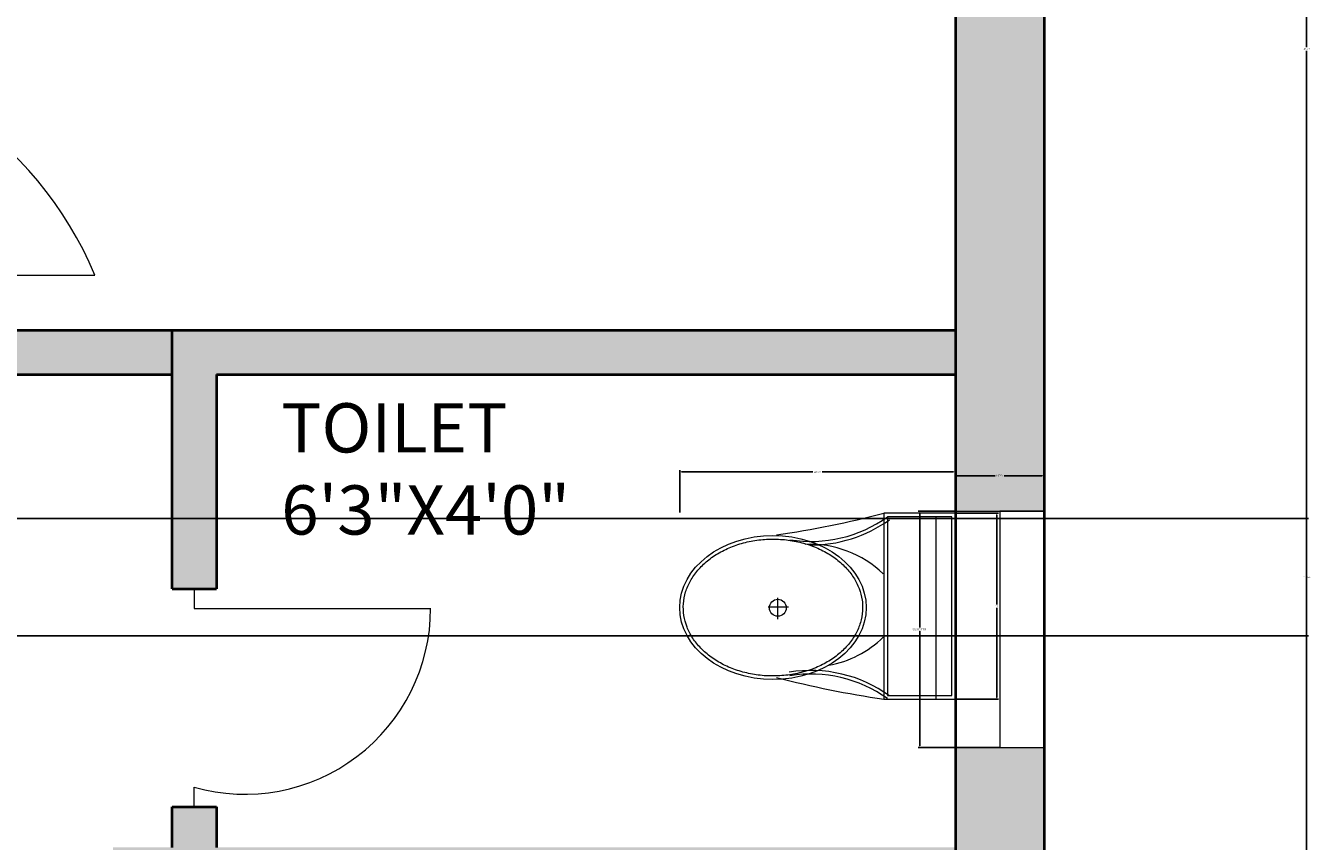
# Model space of a CAD drawing. Units: inches. Extents: x 1441 to 2460, y 1648 to 2683.
# Tile 14 of 35: x 1786 to 1916, y 1975 to 2058. Entities that reach past the tile are written whole.
import ezdxf

# ---------------------------------------------------------------- set-up
doc = ezdxf.new("R2010")
doc.units = ezdxf.units.IN
for name, color, linetype, lineweight in [('A-ANNO-DIMS', 2, 'Continuous', 18), ('A-AREA-IDEN', 7, 'Continuous', 20), ('A-DOOR', 3, 'Continuous', 20), ('A-FLOR-FIXT', 9, 'Continuous', 18), ('A-GLAZ', 4, 'Continuous', 18), ('A-WALL', 7, 'Continuous', 40)]:
    doc.layers.add(name, color=color, linetype=linetype, lineweight=lineweight)
doc.layers.add('A-WALL-PATT', color=251, linetype='Continuous', lineweight=13, true_color=0x636466)
doc.styles.get("Standard").update_dxf_attribs({"font": 'arial.ttf'})
doc.dimstyles.get("Standard").update_dxf_attribs({"dimtxt": 0.18, "dimasz": 0.18, "dimexe": 0.18, "dimexo": 0.0625, "dimgap": 0.09, "dimtad": 0, "dimtih": 1, "dimtoh": 1, "dimdec": 4, "dimzin": 0, "dimdsep": 46, "dimtxsty": 'Standard', "dimcen": 0.09, "dimadec": 0, "dimazin": 0, "dimtfac": 1, "dimtdec": 4, "dimtofl": 0, "dimtmove": 0, "dimatfit": 3, "dimfxl": 1, "dimtolj": 1, "dimtzin": 0, "dimarcsym": 0})

# ---------------------------------------------------------------- blocks, each defined once
blk = doc.blocks.new('A$C31115884')
for p, q in [((257.5, 466.4), (257.5, 523.2)), ((283.1, 497.7), (223.4, 497.7)), ((0, 200), (0, 0)), ((520, 200), (0, 200)), ((10, 190), (10, 10)), ((510, 190), (10, 190)), ((510, 10), (510, 190)), ((520, 0), (520, 200)), ((510, 54.5), (0, 54.5)), ((10, 10), (510, 10)), ((0, 0), (520, 0))]:
    blk.add_line(p, q)
blk.add_circle((255.6, 496.4), 23.6)
for centre, radius, start, end in [((2777.7, -204.6), 2807, 165.4549, 171.7133), ((3237, 905), 2807, 188.2867, 194.5451), ((-294.5, 403.3), 364.7, 324.2091, 9.3499), ((-294.5, 403.3), 374.7, 324.2091, 9.3499), ((805.8, 403.3), 364.7, 170.6501, 215.7909), ((139.5, 406.2), 293.5, 315.8436, 2.6563), ((805.8, 403.3), 374.7, 179.2036, 215.7909), ((383.6, 406.2), 293.5, 190.2774, 224.1564)]:
    blk.add_arc(centre, radius, start, end)
blk.add_ellipse((256.2, 509.9), major_axis=(0, -260.7), ratio=0.772727)
blk.add_open_spline([(256.2, 259.2), (263.1, 259.2), (270, 259.7), (287.8, 262.3), (298.7, 265.1), (319.9, 273.1), (330.2, 278.4), (350.1, 291.1), (359.7, 298.7), (377.7, 315.9), (386.2, 325.5), (401.7, 346.6), (408.8, 358.1), (421.3, 382.5), (426.8, 395.5), (435.9, 422.4), (439.5, 436.4), (444.8, 465.1), (446.5, 479.7), (447.9, 509.2), (447.6, 524), (445, 553.3), (442.7, 567.8), (436.3, 596), (432.1, 609.7), (421.9, 636), (416, 648.6), (402.5, 672.1), (395, 683), (378.6, 703), (369.8, 712.1), (351.1, 728), (341.3, 734.8), (320.9, 746.2), (310.4, 750.7), (288.9, 757.3), (278, 759.4), (256, 761), (245, 760.6), (223.1, 757.2), (212.3, 754.3), (191.1, 746.1), (180.8, 740.7), (160.9, 727.8), (151.4, 720.1), (133.5, 702.7), (125.1, 693), (109.6, 671.7), (102.6, 660.2), (90.2, 635.7), (84.9, 622.7), (76, 595.6), (72.4, 581.6), (67.2, 552.9), (65.6, 538.2), (64.4, 508.8), (64.8, 494), (67.5, 464.7), (69.9, 450.2), (76.6, 422), (80.8, 408.3), (91.1, 382.2), (97.2, 369.7), (110.8, 346.3), (118.4, 335.4), (134.8, 315.6), (143.7, 306.7), (162.4, 290.9), (172.3, 284.2), (192.8, 273), (203.3, 268.6), (224.8, 262.2), (235.8, 260.2), (249.9, 259.3), (253, 259.2), (256.2, 259.2)], degree=3, knots=[0, 0, 0, 0, 0.110105, 0.110105, 0.285049, 0.285049, 0.459994, 0.459994, 0.634938, 0.634938, 0.809882, 0.809882, 0.984827, 0.984827, 1.159771, 1.159771, 1.334715, 1.334715, 1.50966, 1.50966, 1.684604, 1.684604, 1.859549, 1.859549, 2.034493, 2.034493, 2.209437, 2.209437, 2.384382, 2.384382, 2.559326, 2.559326, 2.73427, 2.73427, 2.909215, 2.909215, 3.084159, 3.084159, 3.259103, 3.259103, 3.434048, 3.434048, 3.608992, 3.608992, 3.783936, 3.783936, 3.958881, 3.958881, 4.133825, 4.133825, 4.30877, 4.30877, 4.483714, 4.483714, 4.658658, 4.658658, 4.833603, 4.833603, 5.008547, 5.008547, 5.183491, 5.183491, 5.358436, 5.358436, 5.53338, 5.53338, 5.708324, 5.708324, 5.883269, 5.883269, 6.058213, 6.058213, 6.233158, 6.233158, 6.283185, 6.283185, 6.283185, 6.283185])
blk = doc.blocks.new('DOOR-BED2-30')
for p, q in [((0, 27.22), (0, 25.22)), ((0, 0), (0, 2)), ((0, 2), (4.91, 2)), ((4.91, 2), (34.91, 2))]:
    blk.add_line(p, q)
blk.add_arc((0, -12.65), 37.87, 22.7676, 90)
blk = doc.blocks.new('DOOR-WC-SOUTH-24')
for p, q in [((0, 22.15), (0, 20.15)), ((0, 20.15), (24, 20.15)), ((0, 0), (0, 2))]:
    blk.add_line(p, q)
blk.add_arc((5.13, 20.15), 18.86, 254.1904, 0)
blk = doc.blocks.new('WIN-24-SASH')
for p, q in [((9, 24), (4.5, 24)), ((4.5, 24), (4.5, 0)), ((4.5, 0), (0, 0))]:
    blk.add_line(p, q)
blk = doc.blocks.new('*D32')
at = {"layer": 'A-ANNO-DIMS', "color": 0, "lineweight": -2, "transparency": 16777216}
for p, q in [((1852.41, 2008.68), (1852.41, 2013)), ((1852.59, 2012.82), (1865.93, 2012.82)), ((1880.21, 2012.82), (1866.87, 2012.82)), ((1880.39, 2008.68), (1880.39, 2013))]:
    blk.add_line(p, q, dxfattribs=at)
at = {"layer": 'A-ANNO-DIMS', "color": 0, "transparency": 16777216}
for points in [[(1852.59, 2012.85), (1852.59, 2012.79), (1852.41, 2012.82)], [(1880.21, 2012.85), (1880.21, 2012.79), (1880.39, 2012.82)]]:
    blk.add_solid(points, dxfattribs=at)
at = {"layer": 'Defpoints', "color": 0, "transparency": 16777216}
for p in [(1852.41, 2012.82), (1852.41, 2008.62), (1880.39, 2008.62)]:
    blk.add_point(p, dxfattribs=at)
at = {"layer": 'A-ANNO-DIMS', "color": 0, "transparency": 16777216, "insert": (1866.4, 2012.82), "char_height": 0.18, "attachment_point": 5}
blk.add_mtext('\\A1;WC 28', dxfattribs=at)
blk = doc.blocks.new('*D33')
at = {"layer": 'A-ANNO-DIMS', "color": 0, "lineweight": -2, "transparency": 16777216}
for p, q in [((1880.45, 2008.62), (1884.76, 2008.62)), ((1884.58, 2008.44), (1884.58, 1999.36)), ((1884.58, 1989.92), (1884.58, 1999)), ((1880.45, 1989.74), (1884.76, 1989.74))]:
    blk.add_line(p, q, dxfattribs=at)
at = {"layer": 'A-ANNO-DIMS', "color": 0, "transparency": 16777216}
for points in [[(1884.55, 2008.44), (1884.61, 2008.44), (1884.58, 2008.62)], [(1884.55, 1989.92), (1884.61, 1989.92), (1884.58, 1989.74)]]:
    blk.add_solid(points, dxfattribs=at)
at = {"layer": 'Defpoints', "color": 0, "transparency": 16777216}
for p in [(1880.39, 2008.62), (1884.58, 2008.62), (1880.39, 1989.74)]:
    blk.add_point(p, dxfattribs=at)
at = {"layer": 'A-ANNO-DIMS', "color": 0, "transparency": 16777216, "insert": (1884.58, 1999.18), "char_height": 0.18, "attachment_point": 5}
blk.add_mtext('\\A1;19', dxfattribs=at)
blk = doc.blocks.new('*D60')
at = {"layer": 'A-ANNO-DIMS', "color": 0, "lineweight": -2, "transparency": 16777216}
for p, q in [((1880.32, 2008.83), (1876.61, 2008.83)), ((1876.79, 2008.65), (1876.79, 1997.01)), ((1876.79, 1985.01), (1876.79, 1996.65)), ((1880.32, 1984.83), (1876.61, 1984.83))]:
    blk.add_line(p, q, dxfattribs=at)
at = {"layer": 'A-ANNO-DIMS', "color": 0, "transparency": 16777216}
for points in [[(1876.76, 2008.65), (1876.82, 2008.65), (1876.79, 2008.83)], [(1876.76, 1985.01), (1876.82, 1985.01), (1876.79, 1984.83)]]:
    blk.add_solid(points, dxfattribs=at)
at = {"layer": 'Defpoints', "color": 0, "transparency": 16777216}
for p in [(1876.79, 2008.83), (1880.39, 2008.83), (1880.39, 1984.83)]:
    blk.add_point(p, dxfattribs=at)
at = {"layer": 'A-ANNO-DIMS', "color": 0, "transparency": 16777216, "insert": (1876.79, 1996.83), "char_height": 0.18, "attachment_point": 5}
blk.add_mtext('\\A1;SASH 24 TYP.', dxfattribs=at)
blk = doc.blocks.new('*D61')
at = {"layer": 'A-ANNO-DIMS', "color": 0, "lineweight": -2, "transparency": 16777216}
for p, q in [((1880.39, 2008.89), (1880.39, 2012.61)), ((1880.57, 2012.43), (1884.43, 2012.43)), ((1889.21, 2012.43), (1885.34, 2012.43)), ((1889.39, 2008.89), (1889.39, 2012.61))]:
    blk.add_line(p, q, dxfattribs=at)
at = {"layer": 'A-ANNO-DIMS', "color": 0, "transparency": 16777216}
for points in [[(1880.57, 2012.46), (1880.57, 2012.4), (1880.39, 2012.43)], [(1889.21, 2012.46), (1889.21, 2012.4), (1889.39, 2012.43)]]:
    blk.add_solid(points, dxfattribs=at)
at = {"layer": 'Defpoints', "color": 0, "transparency": 16777216}
for p in [(1889.39, 2012.43), (1880.39, 2008.83), (1889.39, 2008.83)]:
    blk.add_point(p, dxfattribs=at)
at = {"layer": 'A-ANNO-DIMS', "color": 0, "transparency": 16777216, "insert": (1884.89, 2012.43), "char_height": 0.18, "attachment_point": 5}
blk.add_mtext('\\A1;9 TYP.', dxfattribs=at)
blk = doc.blocks.new('*D67')
at = {"layer": 'A-ANNO-DIMS', "color": 0, "lineweight": -2, "transparency": 16777216}
for p, q in [((1889.45, 2298.7), (1916.22, 2298.7)), ((1916.04, 2298.52), (1916.04, 2055.94)), ((1916.04, 1813), (1916.04, 2055.57)), ((1758.22, 1812.82), (1916.22, 1812.82))]:
    blk.add_line(p, q, dxfattribs=at)
at = {"layer": 'A-ANNO-DIMS', "color": 0, "transparency": 16777216}
for points in [[(1916.01, 2298.52), (1916.07, 2298.52), (1916.04, 2298.7)], [(1916.01, 1813), (1916.07, 1813), (1916.04, 1812.82)]]:
    blk.add_solid(points, dxfattribs=at)
at = {"layer": 'Defpoints', "color": 0, "transparency": 16777216}
for p in [(1889.39, 2298.7), (1916.04, 2298.7), (1758.16, 1812.82)]:
    blk.add_point(p, dxfattribs=at)
at = {"layer": 'A-ANNO-DIMS', "color": 0, "transparency": 16777216, "insert": (1916.04, 2055.76), "char_height": 0.18, "attachment_point": 5}
blk.add_mtext('\\A1;485.9', dxfattribs=at)
blk = doc.blocks.new('*D125')
at = {"layer": 'A-ANNO-DIMS', "color": 0, "lineweight": -2, "transparency": 16777216}
for p, q in [((1616.11, 2008.09), (1916.22, 2008.09)), ((1916.04, 2007.91), (1916.04, 2002.31)), ((1916.04, 1996.35), (1916.04, 2001.95)), ((1616.11, 1996.17), (1916.22, 1996.17))]:
    blk.add_line(p, q, dxfattribs=at)
at = {"layer": 'A-ANNO-DIMS', "color": 0, "transparency": 16777216}
for points in [[(1916.01, 2007.91), (1916.07, 2007.91), (1916.04, 2008.09)], [(1916.01, 1996.35), (1916.07, 1996.35), (1916.04, 1996.17)]]:
    blk.add_solid(points, dxfattribs=at)
at = {"layer": 'Defpoints', "color": 0, "transparency": 16777216}
for p in [(1616.05, 2008.09), (1916.04, 2008.09), (1616.05, 1996.17)]:
    blk.add_point(p, dxfattribs=at)
at = {"layer": 'A-ANNO-DIMS', "color": 0, "transparency": 16777216, "insert": (1916.04, 2002.13), "char_height": 0.18, "attachment_point": 5}
blk.add_mtext('\\A1;11.922', dxfattribs=at)

msp = doc.modelspace()

# ---------------------------------------------------------------- hatches: boundary and pattern name
at = {"layer": 'A-WALL-PATT'}
h = msp.add_hatch(color=256, dxfattribs=at)
h.dxf.hatch_style = 1
h.paths.add_polyline_path([(1627.5085, 2298.6952), (1568.8859, 2298.6952), (1568.8859, 2246.9605), (1577.8859, 2246.9605), (1577.8859, 2289.6952), (1627.5085, 2289.6952), (1627.5085, 2294.1952)])
h.paths.add_polyline_path([(1675.5777, 2298.6952), (1651.5085, 2298.6952), (1651.5085, 2289.6952), (1675.5777, 2289.6952), (1675.5777, 2294.1952)])
h.paths.add_polyline_path([(1667.3859, 2289.6952), (1662.8859, 2289.6952), (1662.8859, 2233.0622), (1667.3859, 2233.0622)])
h.paths.add_polyline_path([(1715.8721, 2294.3362), (1715.8721, 2295.2788), (1715.8721, 2298.6952), (1699.5777, 2298.6952), (1699.5777, 2289.6952), (1715.8721, 2289.6952)])
h.paths.add_polyline_path([(1707.8859, 2289.6952), (1703.3859, 2289.6952), (1703.3859, 2199.6952), (1707.8859, 2199.6952)])
h.paths.add_polyline_path([(1760.3859, 2204.637), (1755.8859, 2204.637), (1755.8859, 2199.6952), (1667.3859, 2199.6952), (1667.3859, 2204.637), (1662.8859, 2204.637), (1662.8859, 2195.1952), (1760.3859, 2195.1952)])
h.paths.add_polyline_path([(1760.3859, 2289.6952), (1755.8859, 2289.6952), (1755.8859, 2233.0622), (1760.3859, 2233.0622)])
h.paths.add_polyline_path([(1889.3859, 2298.6952), (1739.8721, 2298.6952), (1739.8721, 2289.6952), (1880.3859, 2289.6952), (1880.3859, 2250.8051), (1889.3859, 2250.8051)])
h.paths.add_polyline_path([(1889.3859, 2202.8051), (1880.3859, 2202.8051), (1880.3859, 2157.6952), (1747.948, 2157.6952), (1747.948, 2153.1952), (1755.8859, 2153.1952), (1755.8859, 2058.005), (1760.3859, 2058.005), (1760.3859, 2153.1952), (1880.3859, 2153.1952), (1880.3859, 2124.108), (1889.3859, 2124.108)])
h.paths.add_polyline_path([(1889.3859, 1984.8305), (1880.3859, 1984.8305), (1880.3859, 1834.1952), (1889.3859, 1834.1952)])
h.paths.add_polyline_path([(1889.3859, 2076.108), (1880.3859, 2076.108), (1880.3859, 2008.8305), (1889.3859, 2008.8305)])
h.paths.add_polyline_path([(1880.3859, 2027.1952), (1800.8859, 2027.1952), (1800.8859, 2000.9452), (1805.3859, 2000.9452), (1805.3859, 2022.6952), (1880.3859, 2022.6952)])
h.paths.add_polyline_path([(1800.8859, 2027.1952), (1760.3859, 2027.1952), (1760.3859, 2030.7912), (1755.8859, 2030.7912), (1755.8859, 2022.6952), (1800.8859, 2022.6952)])
h.paths.add_polyline_path([(1880.3859, 1974.6952), (1805.3859, 1974.6952), (1805.3859, 1978.7973), (1800.8859, 1978.7973), (1800.8859, 1974.6952), (1794.8823, 1974.6952), (1794.8823, 1970.1952), (1800.8859, 1970.1952), (1805.3859, 1970.1952), (1880.3859, 1970.1952)])
h.paths.add_polyline_path([(1760.3859, 1974.6952), (1755.8859, 1974.6952), (1755.8859, 1925.6952), (1751.8616, 1925.6952), (1751.8616, 1921.1952), (1760.3859, 1921.1952)])
h.paths.add_polyline_path([(1760.3859, 1921.1952), (1755.8859, 1921.1952), (1755.8859, 1843.1952), (1760.3859, 1843.1952)])
h.paths.add_polyline_path([(1799.1136, 1838.6952), (1799.1136, 1843.1952), (1760.3859, 1843.1952), (1751.8944, 1843.1952), (1751.8944, 1834.1952), (1758.1615, 1834.1952), (1799.1136, 1834.1952)])
h.paths.add_polyline_path([(1880.3859, 1843.1952), (1859.1136, 1843.1952), (1859.1136, 1834.1952), (1880.3859, 1834.1952)])
h.paths.add_polyline_path([(1577.8859, 1857.7914), (1568.8859, 1857.7914), (1568.8859, 1834.1952), (1695.0034, 1834.1952), (1695.0034, 1838.6952), (1695.0034, 1843.1952), (1577.8859, 1843.1952)])
h.paths.add_polyline_path([(1577.8859, 1959.2399), (1573.3859, 1959.2399), (1568.8859, 1959.2399), (1568.8859, 1905.7914), (1577.8859, 1905.7914), (1577.8859, 1921.1952), (1703.3859, 1921.1952), (1707.8859, 1921.1952), (1715.1501, 1921.1952), (1715.1501, 1925.6952), (1707.8859, 1925.6952), (1703.3859, 1925.6952), (1577.8859, 1925.6952)])
h.paths.add_polyline_path([(1577.8859, 2106.6907), (1568.8859, 2106.6907), (1568.8859, 2019.2399), (1577.8859, 2019.2399)])
h.paths.add_polyline_path([(1707.8859, 2051.6952), (1703.3859, 2051.6952), (1703.3859, 2048.6952), (1703.3859, 1925.6952), (1707.8859, 1925.6952)])
h.paths.add_polyline_path([(1703.3859, 2051.6952), (1676.3859, 2051.6952), (1676.3859, 2048.6952), (1703.3859, 2048.6952)])
h.paths.add_polyline_path([(1703.3859, 2102.6952), (1676.3859, 2102.6952), (1676.3859, 2099.6952), (1685.3859, 2099.6952), (1703.3859, 2099.6952)])
h.paths.add_polyline_path([(1707.8859, 2153.1952), (1710.5611, 2153.1952), (1710.5611, 2157.6952), (1707.8859, 2157.6952), (1707.8859, 2195.1952), (1703.3859, 2195.1952), (1703.3859, 2099.6952), (1707.8859, 2099.6952)])
h.paths.add_polyline_path([(1577.8859, 2198.9605), (1568.8859, 2198.9605), (1568.8859, 2166.6907), (1577.8859, 2166.6907)])

# ---------------------------------------------------------------- linework, layer by layer
at = {"layer": 'A-GLAZ'}
for p, q in [((1880.3859, 2008.8305), (1889.3859, 2008.8305)), ((1880.3859, 1984.8305), (1889.3859, 1984.8305))]:
    msp.add_line(p, q, dxfattribs=at)
at = {"layer": 'A-WALL'}
for p, q in [((1889.3859, 2298.6952), (1889.3859, 1834.1952)), ((1880.3859, 2153.1952), (1880.3859, 1834.1952)), ((1760.3859, 2027.1952), (1880.3859, 2027.1952)), ((1800.8859, 2000.9452), (1800.8859, 2027.1952)), ((1755.8859, 2022.6952), (1800.8859, 2022.6952)), ((1805.3859, 2022.6952), (1805.3859, 2000.9452)), ((1805.3859, 2022.6952), (1880.3859, 2022.6952)), ((1800.8859, 2000.9452), (1805.3859, 2000.9452)), ((1800.8859, 1974.6952), (1800.8859, 1978.7973)), ((1800.8859, 1978.7973), (1800.8859, 1978.7973)), ((1800.8859, 1978.7973), (1805.3859, 1978.7973)), ((1805.3859, 1978.7973), (1805.3859, 1974.6952))]:
    msp.add_line(p, q, dxfattribs=at)

# ---------------------------------------------------------------- block references
at = {"layer": 'A-DOOR'}
for name, p in [('DOOR-BED2-30', (1758.14, 2030.79)), ('DOOR-WC-SOUTH-24', (1803.14, 1978.8))]:
    msp.add_blockref(name, p, dxfattribs=at)
at = {"layer": 'A-FLOR-FIXT', "xscale": 0.0363005458959751, "yscale": 0.0363005458959751, "zscale": 0.0363005458959751, "rotation": 89.99999999999996}
msp.add_blockref('A$C31115884', (1880.3859, 1989.7444), dxfattribs=at)
at = {"layer": 'A-GLAZ'}
msp.add_blockref('WIN-24-SASH', (1880.39, 1984.83), dxfattribs=at)

# ---------------------------------------------------------------- texts
at = {"layer": 'A-AREA-IDEN', "insert": (1811.9751, 2019.7839), "char_height": 5, "attachment_point": 1}
msp.add_mtext_dynamic_manual_height_columns('TOILET\\P6\'3"X4\'0"', width=85.554017, gutter_width=12.5, heights=[0], dxfattribs=at)

# ---------------------------------------------------------------- dimensions: what is measured, and where the dimension line sits
at = {"layer": 'A-ANNO-DIMS'}
for base, p1, p2, override, picture, middle in [((1916.0359, 2298.6952), (1758.1615, 1812.8171), (1889.3859, 2298.6952), {"dimdec": 1, "dimlfac": 1, "dimrnd": 0, "dimzin": 0, "dimdsep": 46, "dimlunit": 2}, '*D67', (1916.0359, 2055.7561)), ((1916.0359, 2008.0936), (1616.0509, 1996.172), (1616.0509, 2008.0936), {"dimdec": 3, "dimlfac": 1, "dimrnd": 0, "dimzin": 0, "dimdsep": 46, "dimlunit": 2}, '*D125', (1916.0359, 2002.1328)), ((1884.5817, 2008.6207), (1880.3859, 1989.7444), (1880.3859, 2008.6207), {"dimdec": 0, "dimlfac": 1, "dimrnd": 0, "dimzin": 0, "dimdsep": 46, "dimlunit": 2}, '*D33', (1884.5817, 1999.1825))]:
    dim = msp.add_linear_dim(base=base, p1=p1, p2=p2, angle=90, dimstyle='Standard', override=override, dxfattribs=at)
    dim.commit()
    dim.dimension.update_dxf_attribs({"geometry": picture, "text_midpoint": middle})
for base, p1, p2, angle, text, picture, middle in [((1852.4138, 2012.8165), (1880.3859, 2008.6207), (1852.4138, 2008.6207), 180, 'WC <>', '*D32', (1866.3999, 2012.8165)), ((1876.7859, 2008.8305), (1880.3859, 1984.8305), (1880.3859, 2008.8305), 90, 'SASH <> TYP.', '*D60', (1876.7859, 1996.8305))]:
    dim = msp.add_linear_dim(base=base, p1=p1, p2=p2, angle=angle, text=text, dimstyle='Standard', override={"dimdec": 0, "dimlfac": 1, "dimrnd": 0, "dimzin": 0, "dimdsep": 46, "dimlunit": 2}, dxfattribs=at)
    dim.commit()
    dim.dimension.update_dxf_attribs({"geometry": picture, "text_midpoint": middle})
dim = msp.add_linear_dim(base=(1889.3859, 2012.4305), p1=(1880.3859, 2008.8305), p2=(1889.3859, 2008.8305), text='<> TYP.', dimstyle='Standard', override={"dimdec": 0, "dimlfac": 1, "dimrnd": 0, "dimzin": 0, "dimdsep": 46, "dimlunit": 2}, dxfattribs=at)
dim.commit()
dim.dimension.update_dxf_attribs({"geometry": '*D61', "text_midpoint": (1884.8859, 2012.4305)})

doc.saveas('drawing.dxf')
